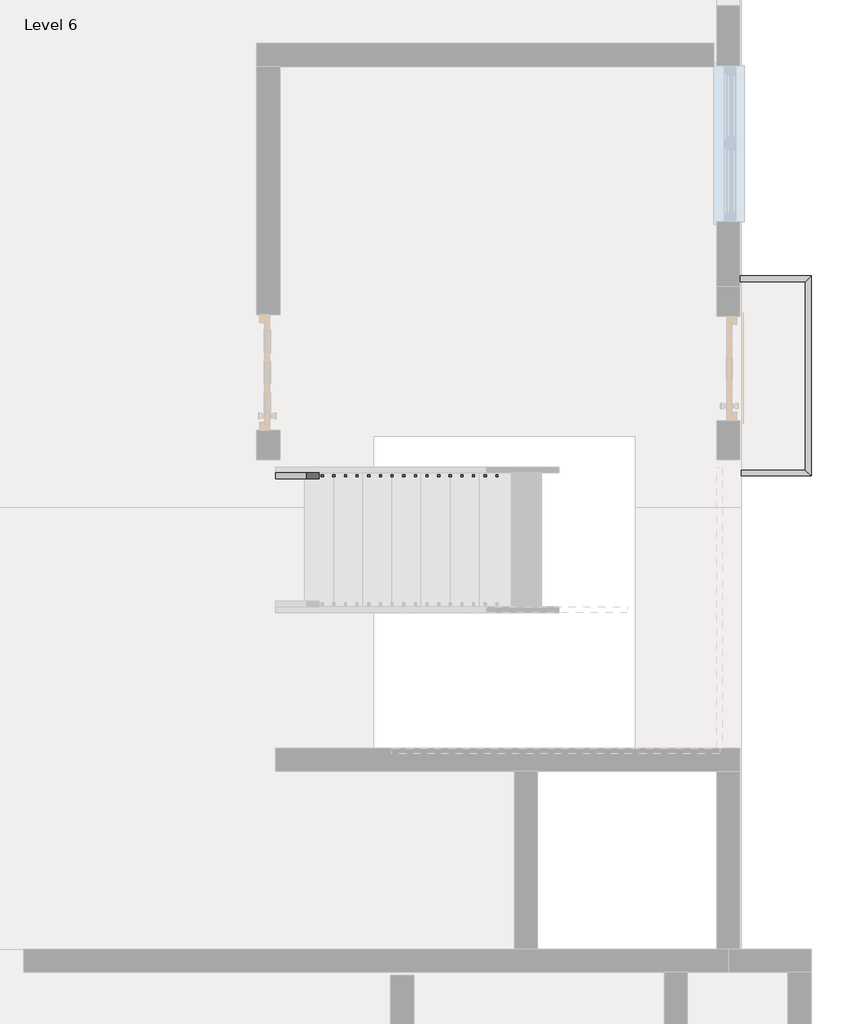
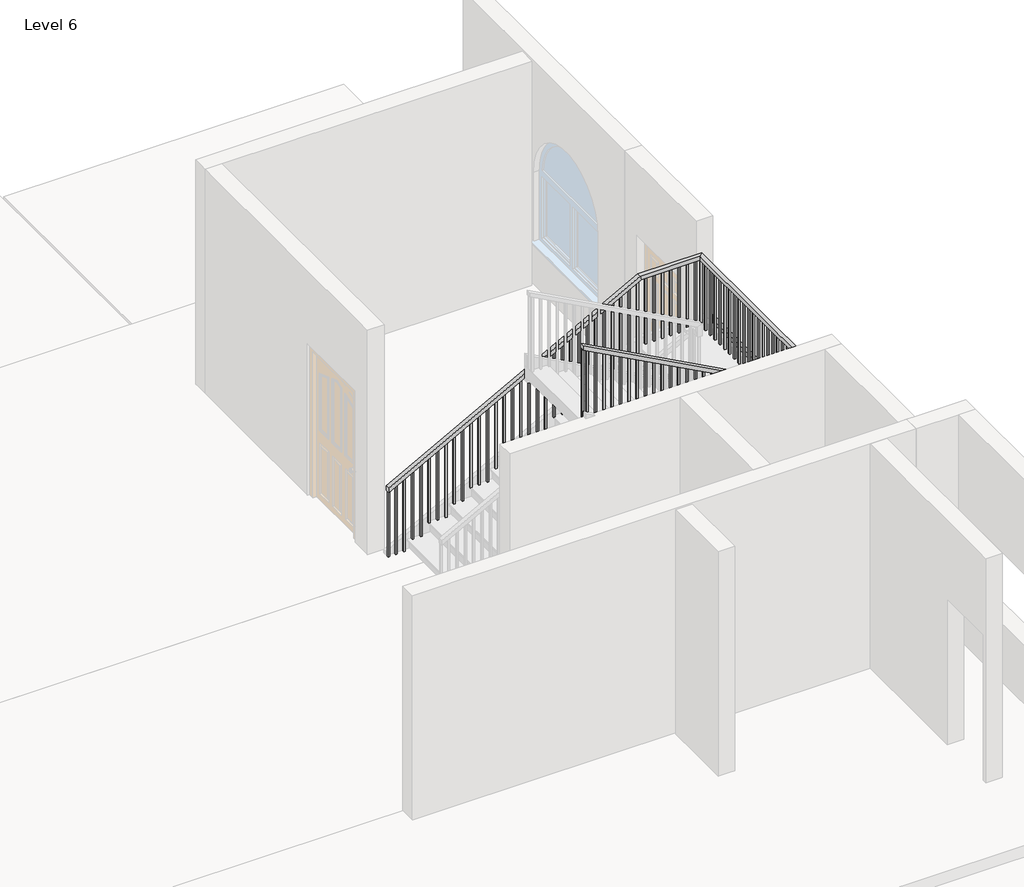
# One storey, part 6 of 7: 2 railings.
"""IFC4 building model written with IfcOpenShell, lengths in millimetres."""

from ifc_helpers import new_model, si_unit, frame, origin, place, context, project, spatial, polyline, outline, extrude, faceted_brep, element, save

model = new_model("IFC4")

# Units and contexts
model_context = context("Model", 3, world=origin())
ifc_project = project(units=[si_unit("LENGTHUNIT", "METRE", prefix="MILLI")], contexts=[model_context])

# Site, building, storey
site = spatial("IfcSite", under=ifc_project)
building = spatial("IfcBuilding", under=site)
storey = spatial("IfcBuildingStorey", under=building, Name="Level 6", Elevation=15240.0)

# Railings
placement = place(None, origin())
element("IfcRailing", 1, ObjectType="Handrail - Rectangular", at=placement, inside=storey, context=model_context, shape_type="SolidModel", body=[
    faceted_brep([(5863.1890963, 3183.81308, 16154.4), (5863.1890963, 3183.81308, 16103.6), (5863.1890963, 3133.01308, 16103.6), (5863.1890963, 3133.01308, 16154.4), (6485.4890963, 3183.81308, 16154.4), (6485.4890963, 3183.81308, 16103.6), (6434.6890963, 3133.01308, 16103.6), (6434.6890963, 3133.01308, 16154.4), (6485.4890963, 1439.3962251, 16154.4), (6485.4890963, 1439.3962251, 16103.6), (6434.6890963, 1490.1962251, 16103.6), (6434.6890963, 1490.1962251, 16154.4), (5875.8890963, 1439.3962251, 16154.4), (5875.8890963, 1490.1962251, 16154.4), (5875.8890963, 1490.1962251, 16103.6), (5875.8890963, 1439.3962251, 16103.6)], [[[0, 1, 2, 3]], [[1, 0, 4, 5]], [[2, 1, 5, 6]], [[3, 2, 6, 7]], [[0, 3, 7, 4]], [[5, 4, 8, 9]], [[6, 5, 9, 10]], [[7, 6, 10, 11]], [[4, 7, 11, 8]], [[12, 13, 14, 15]], [[9, 8, 12, 15]], [[10, 9, 15, 14]], [[11, 10, 14, 13]], [[8, 11, 13, 12]]]),
    extrude(outline(polyline([(5961.6140963, 1474.3212251), (5961.6140963, 1455.2712251), (5942.5640963, 1455.2712251), (5942.5640963, 1474.3212251), (5961.6140963, 1474.3212251)])), frame((0.0, 0.0, 15240.0), z_axis=(0.0, 0.0, 1.0), x_axis=(1.0, 0.0, 0.0)), (0.0, 0.0, 1.0), 863.6),
    extrude(outline(polyline([(6063.2140963, 1474.3212251), (6063.2140963, 1455.2712251), (6044.1640963, 1455.2712251), (6044.1640963, 1474.3212251), (6063.2140963, 1474.3212251)])), frame((0.0, 0.0, 15240.0), z_axis=(0.0, 0.0, 1.0), x_axis=(1.0, 0.0, 0.0)), (0.0, 0.0, 1.0), 863.6),
    extrude(outline(polyline([(6164.8140963, 1474.3212251), (6164.8140963, 1455.2712251), (6145.7640963, 1455.2712251), (6145.7640963, 1474.3212251), (6164.8140963, 1474.3212251)])), frame((0.0, 0.0, 15240.0), z_axis=(0.0, 0.0, 1.0), x_axis=(1.0, 0.0, 0.0)), (0.0, 0.0, 1.0), 863.6),
    extrude(outline(polyline([(6266.4140963, 1474.3212251), (6266.4140963, 1455.2712251), (6247.3640963, 1455.2712251), (6247.3640963, 1474.3212251), (6266.4140963, 1474.3212251)])), frame((0.0, 0.0, 15240.0), z_axis=(0.0, 0.0, 1.0), x_axis=(1.0, 0.0, 0.0)), (0.0, 0.0, 1.0), 863.6),
    extrude(outline(polyline([(6368.0140963, 1474.3212251), (6368.0140963, 1455.2712251), (6348.9640963, 1455.2712251), (6348.9640963, 1474.3212251), (6368.0140963, 1474.3212251)])), frame((0.0, 0.0, 15240.0), z_axis=(0.0, 0.0, 1.0), x_axis=(1.0, 0.0, 0.0)), (0.0, 0.0, 1.0), 863.6),
    extrude(outline(polyline([(6450.5640963, 1542.33808), (6469.6140963, 1542.33808), (6469.6140963, 1523.28808), (6450.5640963, 1523.28808), (6450.5640963, 1542.33808)])), frame((0.0, 0.0, 15240.0), z_axis=(0.0, 0.0, 1.0), x_axis=(1.0, 0.0, 0.0)), (0.0, 0.0, 1.0), 863.6),
    extrude(outline(polyline([(6450.5640963, 1643.93808), (6469.6140963, 1643.93808), (6469.6140963, 1624.88808), (6450.5640963, 1624.88808), (6450.5640963, 1643.93808)])), frame((0.0, 0.0, 15240.0), z_axis=(0.0, 0.0, 1.0), x_axis=(1.0, 0.0, 0.0)), (0.0, 0.0, 1.0), 863.6),
    extrude(outline(polyline([(6450.5640963, 1745.53808), (6469.6140963, 1745.53808), (6469.6140963, 1726.48808), (6450.5640963, 1726.48808), (6450.5640963, 1745.53808)])), frame((0.0, 0.0, 15240.0), z_axis=(0.0, 0.0, 1.0), x_axis=(1.0, 0.0, 0.0)), (0.0, 0.0, 1.0), 863.6),
    extrude(outline(polyline([(6450.5640963, 1847.13808), (6469.6140963, 1847.13808), (6469.6140963, 1828.08808), (6450.5640963, 1828.08808), (6450.5640963, 1847.13808)])), frame((0.0, 0.0, 15240.0), z_axis=(0.0, 0.0, 1.0), x_axis=(1.0, 0.0, 0.0)), (0.0, 0.0, 1.0), 863.6),
    extrude(outline(polyline([(6450.5640963, 1948.73808), (6469.6140963, 1948.73808), (6469.6140963, 1929.68808), (6450.5640963, 1929.68808), (6450.5640963, 1948.73808)])), frame((0.0, 0.0, 15240.0), z_axis=(0.0, 0.0, 1.0), x_axis=(1.0, 0.0, 0.0)), (0.0, 0.0, 1.0), 863.6),
    extrude(outline(polyline([(6450.5640963, 2050.33808), (6469.6140963, 2050.33808), (6469.6140963, 2031.28808), (6450.5640963, 2031.28808), (6450.5640963, 2050.33808)])), frame((0.0, 0.0, 15240.0), z_axis=(0.0, 0.0, 1.0), x_axis=(1.0, 0.0, 0.0)), (0.0, 0.0, 1.0), 863.6),
    extrude(outline(polyline([(6450.5640963, 2151.93808), (6469.6140963, 2151.93808), (6469.6140963, 2132.88808), (6450.5640963, 2132.88808), (6450.5640963, 2151.93808)])), frame((0.0, 0.0, 15240.0), z_axis=(0.0, 0.0, 1.0), x_axis=(1.0, 0.0, 0.0)), (0.0, 0.0, 1.0), 863.6),
    extrude(outline(polyline([(6450.5640963, 2253.53808), (6469.6140963, 2253.53808), (6469.6140963, 2234.48808), (6450.5640963, 2234.48808), (6450.5640963, 2253.53808)])), frame((0.0, 0.0, 15240.0), z_axis=(0.0, 0.0, 1.0), x_axis=(1.0, 0.0, 0.0)), (0.0, 0.0, 1.0), 863.6),
    extrude(outline(polyline([(6450.5640963, 2355.13808), (6469.6140963, 2355.13808), (6469.6140963, 2336.08808), (6450.5640963, 2336.08808), (6450.5640963, 2355.13808)])), frame((0.0, 0.0, 15240.0), z_axis=(0.0, 0.0, 1.0), x_axis=(1.0, 0.0, 0.0)), (0.0, 0.0, 1.0), 863.6),
    extrude(outline(polyline([(6450.5640963, 2456.73808), (6469.6140963, 2456.73808), (6469.6140963, 2437.68808), (6450.5640963, 2437.68808), (6450.5640963, 2456.73808)])), frame((0.0, 0.0, 15240.0), z_axis=(0.0, 0.0, 1.0), x_axis=(1.0, 0.0, 0.0)), (0.0, 0.0, 1.0), 863.6),
    extrude(outline(polyline([(6450.5640963, 2558.33808), (6469.6140963, 2558.33808), (6469.6140963, 2539.28808), (6450.5640963, 2539.28808), (6450.5640963, 2558.33808)])), frame((0.0, 0.0, 15240.0), z_axis=(0.0, 0.0, 1.0), x_axis=(1.0, 0.0, 0.0)), (0.0, 0.0, 1.0), 863.6),
    extrude(outline(polyline([(6450.5640963, 2659.93808), (6469.6140963, 2659.93808), (6469.6140963, 2640.88808), (6450.5640963, 2640.88808), (6450.5640963, 2659.93808)])), frame((0.0, 0.0, 15240.0), z_axis=(0.0, 0.0, 1.0), x_axis=(1.0, 0.0, 0.0)), (0.0, 0.0, 1.0), 863.6),
    extrude(outline(polyline([(6450.5640963, 2761.53808), (6469.6140963, 2761.53808), (6469.6140963, 2742.48808), (6450.5640963, 2742.48808), (6450.5640963, 2761.53808)])), frame((0.0, 0.0, 15240.0), z_axis=(0.0, 0.0, 1.0), x_axis=(1.0, 0.0, 0.0)), (0.0, 0.0, 1.0), 863.6),
    extrude(outline(polyline([(6450.5640963, 2863.13808), (6469.6140963, 2863.13808), (6469.6140963, 2844.08808), (6450.5640963, 2844.08808), (6450.5640963, 2863.13808)])), frame((0.0, 0.0, 15240.0), z_axis=(0.0, 0.0, 1.0), x_axis=(1.0, 0.0, 0.0)), (0.0, 0.0, 1.0), 863.6),
    extrude(outline(polyline([(6450.5640963, 2964.73808), (6469.6140963, 2964.73808), (6469.6140963, 2945.68808), (6450.5640963, 2945.68808), (6450.5640963, 2964.73808)])), frame((0.0, 0.0, 15240.0), z_axis=(0.0, 0.0, 1.0), x_axis=(1.0, 0.0, 0.0)), (0.0, 0.0, 1.0), 863.6),
    extrude(outline(polyline([(6450.5640963, 3066.33808), (6469.6140963, 3066.33808), (6469.6140963, 3047.28808), (6450.5640963, 3047.28808), (6450.5640963, 3066.33808)])), frame((0.0, 0.0, 15240.0), z_axis=(0.0, 0.0, 1.0), x_axis=(1.0, 0.0, 0.0)), (0.0, 0.0, 1.0), 863.6),
    extrude(outline(polyline([(6361.6640963, 3148.88808), (6361.6640963, 3167.93808), (6380.7140963, 3167.93808), (6380.7140963, 3148.88808), (6361.6640963, 3148.88808)])), frame((0.0, 0.0, 15240.0), z_axis=(0.0, 0.0, 1.0), x_axis=(1.0, 0.0, 0.0)), (0.0, 0.0, 1.0), 863.6),
    extrude(outline(polyline([(6260.0640963, 3148.88808), (6260.0640963, 3167.93808), (6279.1140963, 3167.93808), (6279.1140963, 3148.88808), (6260.0640963, 3148.88808)])), frame((0.0, 0.0, 15240.0), z_axis=(0.0, 0.0, 1.0), x_axis=(1.0, 0.0, 0.0)), (0.0, 0.0, 1.0), 863.6),
    extrude(outline(polyline([(6158.4640963, 3148.88808), (6158.4640963, 3167.93808), (6177.5140963, 3167.93808), (6177.5140963, 3148.88808), (6158.4640963, 3148.88808)])), frame((0.0, 0.0, 15240.0), z_axis=(0.0, 0.0, 1.0), x_axis=(1.0, 0.0, 0.0)), (0.0, 0.0, 1.0), 863.6),
    extrude(outline(polyline([(6056.8640963, 3148.88808), (6056.8640963, 3167.93808), (6075.9140963, 3167.93808), (6075.9140963, 3148.88808), (6056.8640963, 3148.88808)])), frame((0.0, 0.0, 15240.0), z_axis=(0.0, 0.0, 1.0), x_axis=(1.0, 0.0, 0.0)), (0.0, 0.0, 1.0), 863.6),
    extrude(outline(polyline([(5955.2640963, 3148.88808), (5955.2640963, 3167.93808), (5974.3140963, 3167.93808), (5974.3140963, 3148.88808), (5955.2640963, 3148.88808)])), frame((0.0, 0.0, 15240.0), z_axis=(0.0, 0.0, 1.0), x_axis=(1.0, 0.0, 0.0)), (0.0, 0.0, 1.0), 863.6),
    extrude(outline(polyline([(6450.5640963, 1474.3212251), (6469.6140963, 1474.3212251), (6469.6140963, 1455.2712251), (6450.5640963, 1455.2712251), (6450.5640963, 1474.3212251)])), frame((0.0, 0.0, 15240.0), z_axis=(0.0, 0.0, 1.0), x_axis=(1.0, 0.0, 0.0)), (0.0, 0.0, 1.0), 863.6),
    extrude(outline(polyline([(6450.5640963, 3148.88808), (6450.5640963, 3167.93808), (6469.6140963, 3167.93808), (6469.6140963, 3148.88808), (6450.5640963, 3148.88808)])), frame((0.0, 0.0, 15240.0), z_axis=(0.0, 0.0, 1.0), x_axis=(1.0, 0.0, 0.0)), (0.0, 0.0, 1.0), 863.6),
    extrude(outline(polyline([(5894.9390963, 1474.3212251), (5894.9390963, 1455.2712251), (5875.8890963, 1455.2712251), (5875.8890963, 1474.3212251), (5894.9390963, 1474.3212251)])), frame((0.0, 0.0, 15240.0), z_axis=(0.0, 0.0, 1.0), x_axis=(1.0, 0.0, 0.0)), (0.0, 0.0, 1.0), 863.6),
    extrude(outline(polyline([(5863.1890963, 3148.88808), (5863.1890963, 3167.93808), (5882.2390963, 3167.93808), (5882.2390963, 3148.88808), (5863.1890963, 3148.88808)])), frame((0.0, 0.0, 15240.0), z_axis=(0.0, 0.0, 1.0), x_axis=(1.0, 0.0, 0.0)), (0.0, 0.0, 1.0), 863.6),
])
element("IfcRailing", 2, ObjectType="Handrail - Rectangular", at=placement, inside=storey, context=model_context, shape_type="SolidModel", body=[
    faceted_brep([(1811.8890963, 1464.7962251, 16292.9454545), (1811.8890963, 1464.7962251, 16235.1709673), (1811.8890963, 1413.9962251, 16235.1709673), (1811.8890963, 1413.9962251, 16292.9454545), (4881.0326586, 1464.7962251, 17955.4909091), (4893.9079172, 1464.7962251, 17904.6909091), (4893.9079172, 1413.9962251, 17904.6909091), (4881.0326586, 1413.9962251, 17955.4909091), (5659.9890963, 1464.7962251, 17955.4909091), (5659.9890963, 1464.7962251, 17904.6909091), (5609.1890963, 1413.9962251, 17904.6909091), (5609.1890963, 1413.9962251, 17955.4909091), (5659.9890963, -935.5037749, 17955.4909091), (5659.9890963, -935.5037749, 17904.6909091), (5609.1890963, -884.7037749, 17904.6909091), (5609.1890963, -884.7037749, 17955.4909091), (5137.6756039, -935.5037749, 17955.4909091), (5124.8392301, -935.5037749, 17904.6909091), (5124.8392301, -884.7037749, 17904.6909091), (5137.6756039, -884.7037749, 17955.4909091), (2827.8890963, -935.5037749, 19202.4), (2827.8890963, -884.7037749, 19202.4), (2827.8890963, -884.7037749, 19144.6704456), (2827.8890963, -935.5037749, 19144.6704456)], [[[0, 1, 2, 3]], [[1, 0, 4, 5]], [[2, 1, 5, 6]], [[3, 2, 6, 7]], [[0, 3, 7, 4]], [[5, 4, 8, 9]], [[6, 5, 9, 10]], [[7, 6, 10, 11]], [[4, 7, 11, 8]], [[9, 8, 12, 13]], [[10, 9, 13, 14]], [[11, 10, 14, 15]], [[8, 11, 15, 12]], [[13, 12, 16, 17]], [[14, 13, 17, 18]], [[15, 14, 18, 19]], [[12, 15, 19, 16]], [[20, 21, 22, 23]], [[17, 16, 20, 23]], [[18, 17, 23, 22]], [[19, 18, 22, 21]], [[16, 19, 21, 20]]]),
    extrude(outline(polyline([(19115.5858236, 2881.8640963), (18149.4545455, 2881.8640963), (18149.4545455, 2900.9140963), (19105.2664983, 2900.9140963), (19115.5858236, 2881.8640963)])), frame((0.0, -919.6287749, 0.0), z_axis=(0.0, 1.0, 0.0), x_axis=(0.0, 0.0, 1.0)), (0.0, 0.0, 1.0), 19.05),
    extrude(outline(polyline([(19060.5494219, 2983.4640963), (18149.4545455, 2983.4640963), (18149.4545455, 3002.5140963), (19050.2300965, 3002.5140963), (19060.5494219, 2983.4640963)])), frame((0.0, -919.6287749, 0.0), z_axis=(0.0, 1.0, 0.0), x_axis=(0.0, 0.0, 1.0)), (0.0, 0.0, 1.0), 19.05),
    extrude(outline(polyline([(19005.8377681, 3085.0640963), (18010.9090909, 3085.0640963), (18010.9090909, 3104.1140963), (18995.553866, 3104.1140963), (19005.8377681, 3085.0640963)])), frame((0.0, -919.6287749, 0.0), z_axis=(0.0, 1.0, 0.0), x_axis=(0.0, 0.0, 1.0)), (0.0, 0.0, 1.0), 19.05),
    extrude(outline(polyline([(18950.9902905, 3186.6640963), (18010.9090909, 3186.6640963), (18010.9090909, 3205.7140963), (18940.7063885, 3205.7140963), (18950.9902905, 3186.6640963)])), frame((0.0, -919.6287749, 0.0), z_axis=(0.0, 1.0, 0.0), x_axis=(0.0, 0.0, 1.0)), (0.0, 0.0, 1.0), 19.05),
    extrude(outline(polyline([(18896.1428129, 3288.2640963), (18010.9090909, 3288.2640963), (18010.9090909, 3307.3140963), (18885.8589109, 3307.3140963), (18896.1428129, 3288.2640963)])), frame((0.0, -919.6287749, 0.0), z_axis=(0.0, 1.0, 0.0), x_axis=(0.0, 0.0, 1.0)), (0.0, 0.0, 1.0), 19.05),
    extrude(outline(polyline([(18841.2953354, 3389.8640963), (17872.3636364, 3389.8640963), (17872.3636364, 3408.9140963), (18831.0114333, 3408.9140963), (18841.2953354, 3389.8640963)])), frame((0.0, -919.6287749, 0.0), z_axis=(0.0, 1.0, 0.0), x_axis=(0.0, 0.0, 1.0)), (0.0, 0.0, 1.0), 19.05),
    extrude(outline(polyline([(18786.4478578, 3491.4640963), (17872.3636364, 3491.4640963), (17872.3636364, 3510.5140963), (18776.1639558, 3510.5140963), (18786.4478578, 3491.4640963)])), frame((0.0, -919.6287749, 0.0), z_axis=(0.0, 1.0, 0.0), x_axis=(0.0, 0.0, 1.0)), (0.0, 0.0, 1.0), 19.05),
    extrude(outline(polyline([(18731.6003803, 3593.0640963), (17733.8181818, 3593.0640963), (17733.8181818, 3612.1140963), (18721.3164782, 3612.1140963), (18731.6003803, 3593.0640963)])), frame((0.0, -919.6287749, 0.0), z_axis=(0.0, 1.0, 0.0), x_axis=(0.0, 0.0, 1.0)), (0.0, 0.0, 1.0), 19.05),
    extrude(outline(polyline([(18676.7529027, 3694.6640963), (17733.8181818, 3694.6640963), (17733.8181818, 3713.7140963), (18666.4690007, 3713.7140963), (18676.7529027, 3694.6640963)])), frame((0.0, -919.6287749, 0.0), z_axis=(0.0, 1.0, 0.0), x_axis=(0.0, 0.0, 1.0)), (0.0, 0.0, 1.0), 19.05),
    extrude(outline(polyline([(18621.9054252, 3796.2640963), (17733.8181818, 3796.2640963), (17733.8181818, 3815.3140963), (18611.6215231, 3815.3140963), (18621.9054252, 3796.2640963)])), frame((0.0, -919.6287749, 0.0), z_axis=(0.0, 1.0, 0.0), x_axis=(0.0, 0.0, 1.0)), (0.0, 0.0, 1.0), 19.05),
    extrude(outline(polyline([(18567.1307062, 3897.8640963), (17595.2727273, 3897.8640963), (17595.2727273, 3916.9140963), (18556.8113809, 3916.9140963), (18567.1307062, 3897.8640963)])), frame((0.0, -919.6287749, 0.0), z_axis=(0.0, 1.0, 0.0), x_axis=(0.0, 0.0, 1.0)), (0.0, 0.0, 1.0), 19.05),
    extrude(outline(polyline([(18512.0943044, 3999.4640963), (17595.2727273, 3999.4640963), (17595.2727273, 4018.5140963), (18501.7749791, 4018.5140963), (18512.0943044, 3999.4640963)])), frame((0.0, -919.6287749, 0.0), z_axis=(0.0, 1.0, 0.0), x_axis=(0.0, 0.0, 1.0)), (0.0, 0.0, 1.0), 19.05),
    extrude(outline(polyline([(18457.3629925, 4101.0640963), (17456.7272727, 4101.0640963), (17456.7272727, 4120.1140963), (18447.0790904, 4120.1140963), (18457.3629925, 4101.0640963)])), frame((0.0, -919.6287749, 0.0), z_axis=(0.0, 1.0, 0.0), x_axis=(0.0, 0.0, 1.0)), (0.0, 0.0, 1.0), 19.05),
    extrude(outline(polyline([(18402.5155149, 4202.6640963), (17456.7272727, 4202.6640963), (17456.7272727, 4221.7140963), (18392.2316129, 4221.7140963), (18402.5155149, 4202.6640963)])), frame((0.0, -919.6287749, 0.0), z_axis=(0.0, 1.0, 0.0), x_axis=(0.0, 0.0, 1.0)), (0.0, 0.0, 1.0), 19.05),
    extrude(outline(polyline([(18347.6680374, 4304.2640963), (17456.7272727, 4304.2640963), (17456.7272727, 4323.3140963), (18337.3841353, 4323.3140963), (18347.6680374, 4304.2640963)])), frame((0.0, -919.6287749, 0.0), z_axis=(0.0, 1.0, 0.0), x_axis=(0.0, 0.0, 1.0)), (0.0, 0.0, 1.0), 19.05),
    extrude(outline(polyline([(18292.8205598, 4405.8640963), (17318.1818182, 4405.8640963), (17318.1818182, 4424.9140963), (18282.5366578, 4424.9140963), (18292.8205598, 4405.8640963)])), frame((0.0, -919.6287749, 0.0), z_axis=(0.0, 1.0, 0.0), x_axis=(0.0, 0.0, 1.0)), (0.0, 0.0, 1.0), 19.05),
    extrude(outline(polyline([(18237.9730823, 4507.4640963), (17318.1818182, 4507.4640963), (17318.1818182, 4526.5140963), (18227.6891802, 4526.5140963), (18237.9730823, 4507.4640963)])), frame((0.0, -919.6287749, 0.0), z_axis=(0.0, 1.0, 0.0), x_axis=(0.0, 0.0, 1.0)), (0.0, 0.0, 1.0), 19.05),
    extrude(outline(polyline([(18183.1256047, 4609.0640963), (17179.6363636, 4609.0640963), (17179.6363636, 4628.1140963), (18172.8417027, 4628.1140963), (18183.1256047, 4609.0640963)])), frame((0.0, -919.6287749, 0.0), z_axis=(0.0, 1.0, 0.0), x_axis=(0.0, 0.0, 1.0)), (0.0, 0.0, 1.0), 19.05),
    extrude(outline(polyline([(18128.2781272, 4710.6640963), (17179.6363636, 4710.6640963), (17179.6363636, 4729.7140963), (18117.9942251, 4729.7140963), (18128.2781272, 4710.6640963)])), frame((0.0, -919.6287749, 0.0), z_axis=(0.0, 1.0, 0.0), x_axis=(0.0, 0.0, 1.0)), (0.0, 0.0, 1.0), 19.05),
    extrude(outline(polyline([(18073.4306496, 4812.2640963), (17179.6363636, 4812.2640963), (17179.6363636, 4831.3140963), (18063.1467476, 4831.3140963), (18073.4306496, 4812.2640963)])), frame((0.0, -919.6287749, 0.0), z_axis=(0.0, 1.0, 0.0), x_axis=(0.0, 0.0, 1.0)), (0.0, 0.0, 1.0), 19.05),
    extrude(outline(polyline([(18018.583172, 4913.8640963), (17041.0909091, 4913.8640963), (17041.0909091, 4932.9140963), (18008.29927, 4932.9140963), (18018.583172, 4913.8640963)])), frame((0.0, -919.6287749, 0.0), z_axis=(0.0, 1.0, 0.0), x_axis=(0.0, 0.0, 1.0)), (0.0, 0.0, 1.0), 19.05),
    extrude(outline(polyline([(17963.7356945, 5015.4640963), (17041.0909091, 5015.4640963), (17041.0909091, 5034.5140963), (17953.4517924, 5034.5140963), (17963.7356945, 5015.4640963)])), frame((0.0, -919.6287749, 0.0), z_axis=(0.0, 1.0, 0.0), x_axis=(0.0, 0.0, 1.0)), (0.0, 0.0, 1.0), 19.05),
    extrude(outline(polyline([(17908.8882169, 5117.0640963), (17041.0909091, 5117.0640963), (17041.0909091, 5136.1140963), (17898.6043149, 5136.1140963), (17908.8882169, 5117.0640963)])), frame((0.0, -919.6287749, 0.0), z_axis=(0.0, 1.0, 0.0), x_axis=(0.0, 0.0, 1.0)), (0.0, 0.0, 1.0), 19.05),
    extrude(outline(polyline([(5237.7140963, -919.6287749), (5218.6640963, -919.6287749), (5218.6640963, -900.5787749), (5237.7140963, -900.5787749), (5237.7140963, -919.6287749)])), frame((0.0, 0.0, 17041.0909091), z_axis=(0.0, 0.0, 1.0), x_axis=(1.0, 0.0, 0.0)), (0.0, 0.0, 1.0), 863.6),
    extrude(outline(polyline([(5339.3140963, -919.6287749), (5320.2640963, -919.6287749), (5320.2640963, -900.5787749), (5339.3140963, -900.5787749), (5339.3140963, -919.6287749)])), frame((0.0, 0.0, 17041.0909091), z_axis=(0.0, 0.0, 1.0), x_axis=(1.0, 0.0, 0.0)), (0.0, 0.0, 1.0), 863.6),
    extrude(outline(polyline([(5440.9140963, -919.6287749), (5421.8640963, -919.6287749), (5421.8640963, -900.5787749), (5440.9140963, -900.5787749), (5440.9140963, -919.6287749)])), frame((0.0, 0.0, 17041.0909091), z_axis=(0.0, 0.0, 1.0), x_axis=(1.0, 0.0, 0.0)), (0.0, 0.0, 1.0), 863.6),
    extrude(outline(polyline([(5542.5140963, -919.6287749), (5523.4640963, -919.6287749), (5523.4640963, -900.5787749), (5542.5140963, -900.5787749), (5542.5140963, -919.6287749)])), frame((0.0, 0.0, 17041.0909091), z_axis=(0.0, 0.0, 1.0), x_axis=(1.0, 0.0, 0.0)), (0.0, 0.0, 1.0), 863.6),
    extrude(outline(polyline([(5644.1140963, -887.8787749), (5644.1140963, -906.9287749), (5625.0640963, -906.9287749), (5625.0640963, -887.8787749), (5644.1140963, -887.8787749)])), frame((0.0, 0.0, 17041.0909091), z_axis=(0.0, 0.0, 1.0), x_axis=(1.0, 0.0, 0.0)), (0.0, 0.0, 1.0), 863.6),
    extrude(outline(polyline([(5644.1140963, -786.2787749), (5644.1140963, -805.3287749), (5625.0640963, -805.3287749), (5625.0640963, -786.2787749), (5644.1140963, -786.2787749)])), frame((0.0, 0.0, 17041.0909091), z_axis=(0.0, 0.0, 1.0), x_axis=(1.0, 0.0, 0.0)), (0.0, 0.0, 1.0), 863.6),
    extrude(outline(polyline([(5644.1140963, -684.6787749), (5644.1140963, -703.7287749), (5625.0640963, -703.7287749), (5625.0640963, -684.6787749), (5644.1140963, -684.6787749)])), frame((0.0, 0.0, 17041.0909091), z_axis=(0.0, 0.0, 1.0), x_axis=(1.0, 0.0, 0.0)), (0.0, 0.0, 1.0), 863.6),
    extrude(outline(polyline([(5644.1140963, -583.0787749), (5644.1140963, -602.1287749), (5625.0640963, -602.1287749), (5625.0640963, -583.0787749), (5644.1140963, -583.0787749)])), frame((0.0, 0.0, 17041.0909091), z_axis=(0.0, 0.0, 1.0), x_axis=(1.0, 0.0, 0.0)), (0.0, 0.0, 1.0), 863.6),
    extrude(outline(polyline([(5644.1140963, -481.4787749), (5644.1140963, -500.5287749), (5625.0640963, -500.5287749), (5625.0640963, -481.4787749), (5644.1140963, -481.4787749)])), frame((0.0, 0.0, 17041.0909091), z_axis=(0.0, 0.0, 1.0), x_axis=(1.0, 0.0, 0.0)), (0.0, 0.0, 1.0), 863.6),
    extrude(outline(polyline([(5644.1140963, -379.8787749), (5644.1140963, -398.9287749), (5625.0640963, -398.9287749), (5625.0640963, -379.8787749), (5644.1140963, -379.8787749)])), frame((0.0, 0.0, 17041.0909091), z_axis=(0.0, 0.0, 1.0), x_axis=(1.0, 0.0, 0.0)), (0.0, 0.0, 1.0), 863.6),
    extrude(outline(polyline([(5644.1140963, -278.2787749), (5644.1140963, -297.3287749), (5625.0640963, -297.3287749), (5625.0640963, -278.2787749), (5644.1140963, -278.2787749)])), frame((0.0, 0.0, 17041.0909091), z_axis=(0.0, 0.0, 1.0), x_axis=(1.0, 0.0, 0.0)), (0.0, 0.0, 1.0), 863.6),
    extrude(outline(polyline([(5644.1140963, -176.6787749), (5644.1140963, -195.7287749), (5625.0640963, -195.7287749), (5625.0640963, -176.6787749), (5644.1140963, -176.6787749)])), frame((0.0, 0.0, 17041.0909091), z_axis=(0.0, 0.0, 1.0), x_axis=(1.0, 0.0, 0.0)), (0.0, 0.0, 1.0), 863.6),
    extrude(outline(polyline([(5644.1140963, -75.0787749), (5644.1140963, -94.1287749), (5625.0640963, -94.1287749), (5625.0640963, -75.0787749), (5644.1140963, -75.0787749)])), frame((0.0, 0.0, 17041.0909091), z_axis=(0.0, 0.0, 1.0), x_axis=(1.0, 0.0, 0.0)), (0.0, 0.0, 1.0), 863.6),
    extrude(outline(polyline([(5644.1140963, 26.5212251), (5644.1140963, 7.4712251), (5625.0640963, 7.4712251), (5625.0640963, 26.5212251), (5644.1140963, 26.5212251)])), frame((0.0, 0.0, 17041.0909091), z_axis=(0.0, 0.0, 1.0), x_axis=(1.0, 0.0, 0.0)), (0.0, 0.0, 1.0), 863.6),
    extrude(outline(polyline([(5644.1140963, 128.1212251), (5644.1140963, 109.0712251), (5625.0640963, 109.0712251), (5625.0640963, 128.1212251), (5644.1140963, 128.1212251)])), frame((0.0, 0.0, 17041.0909091), z_axis=(0.0, 0.0, 1.0), x_axis=(1.0, 0.0, 0.0)), (0.0, 0.0, 1.0), 863.6),
    extrude(outline(polyline([(5644.1140963, 229.7212251), (5644.1140963, 210.6712251), (5625.0640963, 210.6712251), (5625.0640963, 229.7212251), (5644.1140963, 229.7212251)])), frame((0.0, 0.0, 17041.0909091), z_axis=(0.0, 0.0, 1.0), x_axis=(1.0, 0.0, 0.0)), (0.0, 0.0, 1.0), 863.6),
    extrude(outline(polyline([(5644.1140963, 331.3212251), (5644.1140963, 312.2712251), (5625.0640963, 312.2712251), (5625.0640963, 331.3212251), (5644.1140963, 331.3212251)])), frame((0.0, 0.0, 17041.0909091), z_axis=(0.0, 0.0, 1.0), x_axis=(1.0, 0.0, 0.0)), (0.0, 0.0, 1.0), 863.6),
    extrude(outline(polyline([(5644.1140963, 432.9212251), (5644.1140963, 413.8712251), (5625.0640963, 413.8712251), (5625.0640963, 432.9212251), (5644.1140963, 432.9212251)])), frame((0.0, 0.0, 17041.0909091), z_axis=(0.0, 0.0, 1.0), x_axis=(1.0, 0.0, 0.0)), (0.0, 0.0, 1.0), 863.6),
    extrude(outline(polyline([(5644.1140963, 534.5212251), (5644.1140963, 515.4712251), (5625.0640963, 515.4712251), (5625.0640963, 534.5212251), (5644.1140963, 534.5212251)])), frame((0.0, 0.0, 17041.0909091), z_axis=(0.0, 0.0, 1.0), x_axis=(1.0, 0.0, 0.0)), (0.0, 0.0, 1.0), 863.6),
    extrude(outline(polyline([(5644.1140963, 636.1212251), (5644.1140963, 617.0712251), (5625.0640963, 617.0712251), (5625.0640963, 636.1212251), (5644.1140963, 636.1212251)])), frame((0.0, 0.0, 17041.0909091), z_axis=(0.0, 0.0, 1.0), x_axis=(1.0, 0.0, 0.0)), (0.0, 0.0, 1.0), 863.6),
    extrude(outline(polyline([(5644.1140963, 737.7212251), (5644.1140963, 718.6712251), (5625.0640963, 718.6712251), (5625.0640963, 737.7212251), (5644.1140963, 737.7212251)])), frame((0.0, 0.0, 17041.0909091), z_axis=(0.0, 0.0, 1.0), x_axis=(1.0, 0.0, 0.0)), (0.0, 0.0, 1.0), 863.6),
    extrude(outline(polyline([(5644.1140963, 839.3212251), (5644.1140963, 820.2712251), (5625.0640963, 820.2712251), (5625.0640963, 839.3212251), (5644.1140963, 839.3212251)])), frame((0.0, 0.0, 17041.0909091), z_axis=(0.0, 0.0, 1.0), x_axis=(1.0, 0.0, 0.0)), (0.0, 0.0, 1.0), 863.6),
    extrude(outline(polyline([(5644.1140963, 940.9212251), (5644.1140963, 921.8712251), (5625.0640963, 921.8712251), (5625.0640963, 940.9212251), (5644.1140963, 940.9212251)])), frame((0.0, 0.0, 17041.0909091), z_axis=(0.0, 0.0, 1.0), x_axis=(1.0, 0.0, 0.0)), (0.0, 0.0, 1.0), 863.6),
    extrude(outline(polyline([(5644.1140963, 1042.5212251), (5644.1140963, 1023.4712251), (5625.0640963, 1023.4712251), (5625.0640963, 1042.5212251), (5644.1140963, 1042.5212251)])), frame((0.0, 0.0, 17041.0909091), z_axis=(0.0, 0.0, 1.0), x_axis=(1.0, 0.0, 0.0)), (0.0, 0.0, 1.0), 863.6),
    extrude(outline(polyline([(5644.1140963, 1144.1212251), (5644.1140963, 1125.0712251), (5625.0640963, 1125.0712251), (5625.0640963, 1144.1212251), (5644.1140963, 1144.1212251)])), frame((0.0, 0.0, 17041.0909091), z_axis=(0.0, 0.0, 1.0), x_axis=(1.0, 0.0, 0.0)), (0.0, 0.0, 1.0), 863.6),
    extrude(outline(polyline([(5644.1140963, 1245.7212251), (5644.1140963, 1226.6712251), (5625.0640963, 1226.6712251), (5625.0640963, 1245.7212251), (5644.1140963, 1245.7212251)])), frame((0.0, 0.0, 17041.0909091), z_axis=(0.0, 0.0, 1.0), x_axis=(1.0, 0.0, 0.0)), (0.0, 0.0, 1.0), 863.6),
    extrude(outline(polyline([(5644.1140963, 1347.3212251), (5644.1140963, 1328.2712251), (5625.0640963, 1328.2712251), (5625.0640963, 1347.3212251), (5644.1140963, 1347.3212251)])), frame((0.0, 0.0, 17041.0909091), z_axis=(0.0, 0.0, 1.0), x_axis=(1.0, 0.0, 0.0)), (0.0, 0.0, 1.0), 863.6),
    extrude(outline(polyline([(5561.5640963, 1448.9212251), (5580.6140963, 1448.9212251), (5580.6140963, 1429.8712251), (5561.5640963, 1429.8712251), (5561.5640963, 1448.9212251)])), frame((0.0, 0.0, 17041.0909091), z_axis=(0.0, 0.0, 1.0), x_axis=(1.0, 0.0, 0.0)), (0.0, 0.0, 1.0), 863.6),
    extrude(outline(polyline([(5459.9640963, 1448.9212251), (5479.0140963, 1448.9212251), (5479.0140963, 1429.8712251), (5459.9640963, 1429.8712251), (5459.9640963, 1448.9212251)])), frame((0.0, 0.0, 17041.0909091), z_axis=(0.0, 0.0, 1.0), x_axis=(1.0, 0.0, 0.0)), (0.0, 0.0, 1.0), 863.6),
    extrude(outline(polyline([(5358.3640963, 1448.9212251), (5377.4140963, 1448.9212251), (5377.4140963, 1429.8712251), (5358.3640963, 1429.8712251), (5358.3640963, 1448.9212251)])), frame((0.0, 0.0, 17041.0909091), z_axis=(0.0, 0.0, 1.0), x_axis=(1.0, 0.0, 0.0)), (0.0, 0.0, 1.0), 863.6),
    extrude(outline(polyline([(5256.7640963, 1448.9212251), (5275.8140963, 1448.9212251), (5275.8140963, 1429.8712251), (5256.7640963, 1429.8712251), (5256.7640963, 1448.9212251)])), frame((0.0, 0.0, 17041.0909091), z_axis=(0.0, 0.0, 1.0), x_axis=(1.0, 0.0, 0.0)), (0.0, 0.0, 1.0), 863.6),
    extrude(outline(polyline([(5155.1640963, 1448.9212251), (5174.2140963, 1448.9212251), (5174.2140963, 1429.8712251), (5155.1640963, 1429.8712251), (5155.1640963, 1448.9212251)])), frame((0.0, 0.0, 17041.0909091), z_axis=(0.0, 0.0, 1.0), x_axis=(1.0, 0.0, 0.0)), (0.0, 0.0, 1.0), 863.6),
    extrude(outline(polyline([(5053.5640963, 1448.9212251), (5072.6140963, 1448.9212251), (5072.6140963, 1429.8712251), (5053.5640963, 1429.8712251), (5053.5640963, 1448.9212251)])), frame((0.0, 0.0, 17041.0909091), z_axis=(0.0, 0.0, 1.0), x_axis=(1.0, 0.0, 0.0)), (0.0, 0.0, 1.0), 863.6),
    extrude(outline(polyline([(4951.9640963, 1448.9212251), (4971.0140963, 1448.9212251), (4971.0140963, 1429.8712251), (4951.9640963, 1429.8712251), (4951.9640963, 1448.9212251)])), frame((0.0, 0.0, 17041.0909091), z_axis=(0.0, 0.0, 1.0), x_axis=(1.0, 0.0, 0.0)), (0.0, 0.0, 1.0), 863.6),
    extrude(outline(polyline([(17881.1033577, 4850.3640963), (16902.5454545, 4850.3640963), (16902.5454545, 4869.4140963), (17891.422683, 4869.4140963), (17881.1033577, 4850.3640963)])), frame((0.0, 1429.8712251, 0.0), z_axis=(0.0, 1.0, 0.0), x_axis=(0.0, 0.0, 1.0)), (0.0, 0.0, 1.0), 19.05),
    extrude(outline(polyline([(17826.0669559, 4748.7640963), (16902.5454545, 4748.7640963), (16902.5454545, 4767.8140963), (17836.3862812, 4767.8140963), (17826.0669559, 4748.7640963)])), frame((0.0, 1429.8712251, 0.0), z_axis=(0.0, 1.0, 0.0), x_axis=(0.0, 0.0, 1.0)), (0.0, 0.0, 1.0), 19.05),
    extrude(outline(polyline([(17771.0305541, 4647.1640963), (16902.5454545, 4647.1640963), (16902.5454545, 4666.2140963), (17781.3498795, 4666.2140963), (17771.0305541, 4647.1640963)])), frame((0.0, 1429.8712251, 0.0), z_axis=(0.0, 1.0, 0.0), x_axis=(0.0, 0.0, 1.0)), (0.0, 0.0, 1.0), 19.05),
    extrude(outline(polyline([(17715.9941524, 4545.5640963), (16764.0, 4545.5640963), (16764.0, 4564.6140963), (17726.3134777, 4564.6140963), (17715.9941524, 4545.5640963)])), frame((0.0, 1429.8712251, 0.0), z_axis=(0.0, 1.0, 0.0), x_axis=(0.0, 0.0, 1.0)), (0.0, 0.0, 1.0), 19.05),
    extrude(outline(polyline([(17660.9577506, 4443.9640963), (16764.0, 4443.9640963), (16764.0, 4463.0140963), (17671.2770759, 4463.0140963), (17660.9577506, 4443.9640963)])), frame((0.0, 1429.8712251, 0.0), z_axis=(0.0, 1.0, 0.0), x_axis=(0.0, 0.0, 1.0)), (0.0, 0.0, 1.0), 19.05),
    extrude(outline(polyline([(17605.9213488, 4342.3640963), (16764.0, 4342.3640963), (16764.0, 4361.4140963), (17616.2406742, 4361.4140963), (17605.9213488, 4342.3640963)])), frame((0.0, 1429.8712251, 0.0), z_axis=(0.0, 1.0, 0.0), x_axis=(0.0, 0.0, 1.0)), (0.0, 0.0, 1.0), 19.05),
    extrude(outline(polyline([(17550.8849471, 4240.7640963), (16625.4545455, 4240.7640963), (16625.4545455, 4259.8140963), (17561.2042724, 4259.8140963), (17550.8849471, 4240.7640963)])), frame((0.0, 1429.8712251, 0.0), z_axis=(0.0, 1.0, 0.0), x_axis=(0.0, 0.0, 1.0)), (0.0, 0.0, 1.0), 19.05),
    extrude(outline(polyline([(17495.8485453, 4139.1640963), (16625.4545455, 4139.1640963), (16625.4545455, 4158.2140963), (17506.1678706, 4158.2140963), (17495.8485453, 4139.1640963)])), frame((0.0, 1429.8712251, 0.0), z_axis=(0.0, 1.0, 0.0), x_axis=(0.0, 0.0, 1.0)), (0.0, 0.0, 1.0), 19.05),
    extrude(outline(polyline([(17440.8121435, 4037.5640963), (16486.9090909, 4037.5640963), (16486.9090909, 4056.6140963), (17451.1314688, 4056.6140963), (17440.8121435, 4037.5640963)])), frame((0.0, 1429.8712251, 0.0), z_axis=(0.0, 1.0, 0.0), x_axis=(0.0, 0.0, 1.0)), (0.0, 0.0, 1.0), 19.05),
    extrude(outline(polyline([(17385.7757417, 3935.9640963), (16486.9090909, 3935.9640963), (16486.9090909, 3955.0140963), (17396.0950671, 3955.0140963), (17385.7757417, 3935.9640963)])), frame((0.0, 1429.8712251, 0.0), z_axis=(0.0, 1.0, 0.0), x_axis=(0.0, 0.0, 1.0)), (0.0, 0.0, 1.0), 19.05),
    extrude(outline(polyline([(17330.73934, 3834.3640963), (16486.9090909, 3834.3640963), (16486.9090909, 3853.4140963), (17341.0586653, 3853.4140963), (17330.73934, 3834.3640963)])), frame((0.0, 1429.8712251, 0.0), z_axis=(0.0, 1.0, 0.0), x_axis=(0.0, 0.0, 1.0)), (0.0, 0.0, 1.0), 19.05),
    extrude(outline(polyline([(17275.7029382, 3732.7640963), (16348.3636364, 3732.7640963), (16348.3636364, 3751.8140963), (17286.0222635, 3751.8140963), (17275.7029382, 3732.7640963)])), frame((0.0, 1429.8712251, 0.0), z_axis=(0.0, 1.0, 0.0), x_axis=(0.0, 0.0, 1.0)), (0.0, 0.0, 1.0), 19.05),
    extrude(outline(polyline([(17220.6665364, 3631.1640963), (16348.3636364, 3631.1640963), (16348.3636364, 3650.2140963), (17230.9858618, 3650.2140963), (17220.6665364, 3631.1640963)])), frame((0.0, 1429.8712251, 0.0), z_axis=(0.0, 1.0, 0.0), x_axis=(0.0, 0.0, 1.0)), (0.0, 0.0, 1.0), 19.05),
    extrude(outline(polyline([(17165.6301347, 3529.5640963), (16209.8181818, 3529.5640963), (16209.8181818, 3548.6140963), (17175.94946, 3548.6140963), (17165.6301347, 3529.5640963)])), frame((0.0, 1429.8712251, 0.0), z_axis=(0.0, 1.0, 0.0), x_axis=(0.0, 0.0, 1.0)), (0.0, 0.0, 1.0), 19.05),
    extrude(outline(polyline([(17110.5937329, 3427.9640963), (16209.8181818, 3427.9640963), (16209.8181818, 3447.0140963), (17120.9130582, 3447.0140963), (17110.5937329, 3427.9640963)])), frame((0.0, 1429.8712251, 0.0), z_axis=(0.0, 1.0, 0.0), x_axis=(0.0, 0.0, 1.0)), (0.0, 0.0, 1.0), 19.05),
    extrude(outline(polyline([(17055.5573311, 3326.3640963), (16209.8181818, 3326.3640963), (16209.8181818, 3345.4140963), (17065.8766565, 3345.4140963), (17055.5573311, 3326.3640963)])), frame((0.0, 1429.8712251, 0.0), z_axis=(0.0, 1.0, 0.0), x_axis=(0.0, 0.0, 1.0)), (0.0, 0.0, 1.0), 19.05),
    extrude(outline(polyline([(17000.5209294, 3224.7640963), (16071.2727273, 3224.7640963), (16071.2727273, 3243.8140963), (17010.8402547, 3243.8140963), (17000.5209294, 3224.7640963)])), frame((0.0, 1429.8712251, 0.0), z_axis=(0.0, 1.0, 0.0), x_axis=(0.0, 0.0, 1.0)), (0.0, 0.0, 1.0), 19.05),
    extrude(outline(polyline([(16945.4845276, 3123.1640963), (16071.2727273, 3123.1640963), (16071.2727273, 3142.2140963), (16955.8038529, 3142.2140963), (16945.4845276, 3123.1640963)])), frame((0.0, 1429.8712251, 0.0), z_axis=(0.0, 1.0, 0.0), x_axis=(0.0, 0.0, 1.0)), (0.0, 0.0, 1.0), 19.05),
    extrude(outline(polyline([(16890.4481258, 3021.5640963), (15932.7272727, 3021.5640963), (15932.7272727, 3040.6140963), (16900.7674512, 3040.6140963), (16890.4481258, 3021.5640963)])), frame((0.0, 1429.8712251, 0.0), z_axis=(0.0, 1.0, 0.0), x_axis=(0.0, 0.0, 1.0)), (0.0, 0.0, 1.0), 19.05),
    extrude(outline(polyline([(16835.4117241, 2919.9640963), (15932.7272727, 2919.9640963), (15932.7272727, 2939.0140963), (16845.7310494, 2939.0140963), (16835.4117241, 2919.9640963)])), frame((0.0, 1429.8712251, 0.0), z_axis=(0.0, 1.0, 0.0), x_axis=(0.0, 0.0, 1.0)), (0.0, 0.0, 1.0), 19.05),
    extrude(outline(polyline([(16780.3753223, 2818.3640963), (15932.7272727, 2818.3640963), (15932.7272727, 2837.4140963), (16790.6946476, 2837.4140963), (16780.3753223, 2818.3640963)])), frame((0.0, 1429.8712251, 0.0), z_axis=(0.0, 1.0, 0.0), x_axis=(0.0, 0.0, 1.0)), (0.0, 0.0, 1.0), 19.05),
    extrude(outline(polyline([(16725.3389205, 2716.7640963), (15794.1818182, 2716.7640963), (15794.1818182, 2735.8140963), (16735.6582459, 2735.8140963), (16725.3389205, 2716.7640963)])), frame((0.0, 1429.8712251, 0.0), z_axis=(0.0, 1.0, 0.0), x_axis=(0.0, 0.0, 1.0)), (0.0, 0.0, 1.0), 19.05),
    extrude(outline(polyline([(16670.3025188, 2615.1640963), (15794.1818182, 2615.1640963), (15794.1818182, 2634.2140963), (16680.6218441, 2634.2140963), (16670.3025188, 2615.1640963)])), frame((0.0, 1429.8712251, 0.0), z_axis=(0.0, 1.0, 0.0), x_axis=(0.0, 0.0, 1.0)), (0.0, 0.0, 1.0), 19.05),
    extrude(outline(polyline([(16615.266117, 2513.5640963), (15655.6363636, 2513.5640963), (15655.6363636, 2532.6140963), (16625.5854423, 2532.6140963), (16615.266117, 2513.5640963)])), frame((0.0, 1429.8712251, 0.0), z_axis=(0.0, 1.0, 0.0), x_axis=(0.0, 0.0, 1.0)), (0.0, 0.0, 1.0), 19.05),
    extrude(outline(polyline([(16560.2297152, 2411.9640963), (15655.6363636, 2411.9640963), (15655.6363636, 2431.0140963), (16570.5490405, 2431.0140963), (16560.2297152, 2411.9640963)])), frame((0.0, 1429.8712251, 0.0), z_axis=(0.0, 1.0, 0.0), x_axis=(0.0, 0.0, 1.0)), (0.0, 0.0, 1.0), 19.05),
    extrude(outline(polyline([(16505.1933134, 2310.3640963), (15655.6363636, 2310.3640963), (15655.6363636, 2329.4140963), (16515.5126388, 2329.4140963), (16505.1933134, 2310.3640963)])), frame((0.0, 1429.8712251, 0.0), z_axis=(0.0, 1.0, 0.0), x_axis=(0.0, 0.0, 1.0)), (0.0, 0.0, 1.0), 19.05),
    extrude(outline(polyline([(16450.1569117, 2208.7640963), (15517.0909091, 2208.7640963), (15517.0909091, 2227.8140963), (16460.476237, 2227.8140963), (16450.1569117, 2208.7640963)])), frame((0.0, 1429.8712251, 0.0), z_axis=(0.0, 1.0, 0.0), x_axis=(0.0, 0.0, 1.0)), (0.0, 0.0, 1.0), 19.05),
    extrude(outline(polyline([(16395.1205099, 2107.1640963), (15517.0909091, 2107.1640963), (15517.0909091, 2126.2140963), (16405.4398352, 2126.2140963), (16395.1205099, 2107.1640963)])), frame((0.0, 1429.8712251, 0.0), z_axis=(0.0, 1.0, 0.0), x_axis=(0.0, 0.0, 1.0)), (0.0, 0.0, 1.0), 19.05),
    extrude(outline(polyline([(16340.0841081, 2005.5640963), (15378.5454545, 2005.5640963), (15378.5454545, 2024.6140963), (16350.4034335, 2024.6140963), (16340.0841081, 2005.5640963)])), frame((0.0, 1429.8712251, 0.0), z_axis=(0.0, 1.0, 0.0), x_axis=(0.0, 0.0, 1.0)), (0.0, 0.0, 1.0), 19.05),
    extrude(outline(polyline([(16285.0477064, 1903.9640963), (15378.5454545, 1903.9640963), (15378.5454545, 1923.0140963), (16295.3670317, 1923.0140963), (16285.0477064, 1903.9640963)])), frame((0.0, 1429.8712251, 0.0), z_axis=(0.0, 1.0, 0.0), x_axis=(0.0, 0.0, 1.0)), (0.0, 0.0, 1.0), 19.05),
    extrude(outline(polyline([(5644.1140963, -900.5787749), (5644.1140963, -919.6287749), (5625.0640963, -919.6287749), (5625.0640963, -900.5787749), (5644.1140963, -900.5787749)])), frame((0.0, 0.0, 17041.0909091), z_axis=(0.0, 0.0, 1.0), x_axis=(1.0, 0.0, 0.0)), (0.0, 0.0, 1.0), 863.6),
    extrude(outline(polyline([(5625.0640963, 1448.9212251), (5644.1140963, 1448.9212251), (5644.1140963, 1429.8712251), (5625.0640963, 1429.8712251), (5625.0640963, 1448.9212251)])), frame((0.0, 0.0, 17041.0909091), z_axis=(0.0, 0.0, 1.0), x_axis=(1.0, 0.0, 0.0)), (0.0, 0.0, 1.0), 863.6),
    extrude(outline(polyline([(19144.6704456, 2827.8890963), (18149.4545455, 2827.8890963), (18149.4545455, 2846.9390963), (19134.3865436, 2846.9390963), (19144.6704456, 2827.8890963)])), frame((0.0, -919.6287749, 0.0), z_axis=(0.0, 1.0, 0.0), x_axis=(0.0, 0.0, 1.0)), (0.0, 0.0, 1.0), 19.05),
    extrude(outline(polyline([(16235.1709673, 1811.8890963), (15378.5454545, 1811.8890963), (15378.5454545, 1830.9390963), (16245.4902926, 1830.9390963), (16235.1709673, 1811.8890963)])), frame((0.0, 1429.8712251, 0.0), z_axis=(0.0, 1.0, 0.0), x_axis=(0.0, 0.0, 1.0)), (0.0, 0.0, 1.0), 19.05),
])

save(model, "model.ifc")

# Revit data of these elements
# Type "Handrail - Rectangular"
#   Assembly Code = "C2010400"
#   built-in parameter 1008612 = 0.0416667 (stored number, unit not read)
#   built-in parameter 1008611 = 0.0416667 (stored number, unit not read)
#   built-in parameter 1008609 = 0.333333 (stored number, unit not read)
#   built-in parameter 1008604 = 0.166667 (stored number, unit not read)
#   built-in parameter 1008603 = 0.166667 (stored number, unit not read)
#   Railing Height = 3' - 0"
#   built-in parameter 1008630 = 2
#   built-in parameter 1008610 = 2
#   built-in parameter 1008618 = Baluster - Square : 3/4"
# Elements 1, 2 (IfcRailing, "Handrail - Rectangular")
#   Phase Created = New Construction
